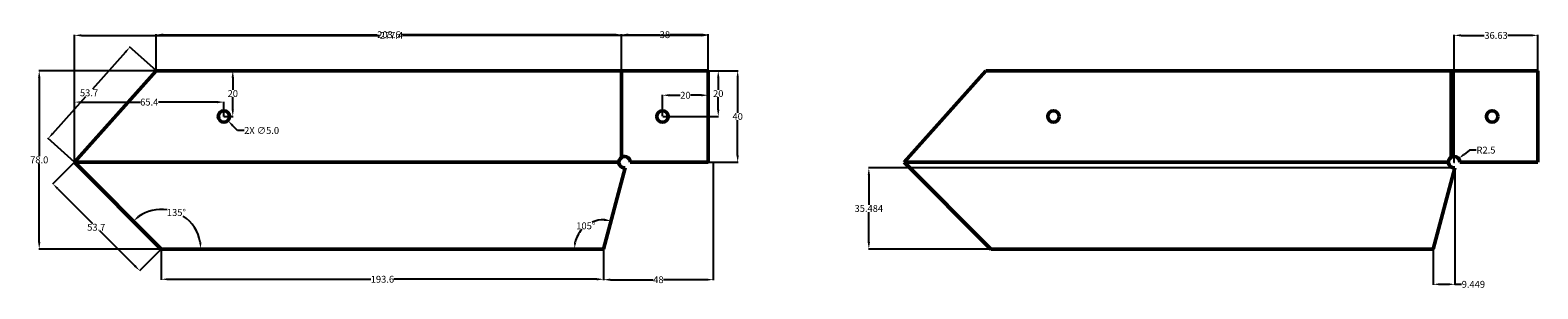
# Model space of a CAD drawing. Units: millimetres. Extents: x -38 to 622, y -14 to 99.
import ezdxf

# ---------------------------------------------------------------- set-up
doc = ezdxf.new("R2010")
doc.units = ezdxf.units.MM
doc.header["$MEASUREMENT"] = 0
doc.layers.add('M-DIMS', color=3, linetype='Continuous', lineweight=25)
doc.layers.add('M-OUTL', color=7, linetype='Continuous', lineweight=50)
doc.styles.get("Standard").update_dxf_attribs({"font": 'arial.ttf'})
doc.dimstyles.get("Standard").update_dxf_attribs({"dimtxt": 3, "dimasz": 3, "dimexe": 0.18, "dimexo": 0.0625, "dimgap": 0.09, "dimtad": 0, "dimtih": 1, "dimtoh": 1, "dimdec": 1, "dimdsep": 46, "dimtxsty": 'Standard', "dimcen": 0.09, "dimadec": 0, "dimazin": 0, "dimtfac": 1, "dimtdec": 1, "dimtofl": 0, "dimtmove": 0, "dimatfit": 3, "dimfxl": 1, "dimtolj": 1, "dimtzin": 0, "dimarcsym": 0})

# ---------------------------------------------------------------- blocks, each defined once
blk = doc.blocks.new('*D1')
at = {"layer": 'Defpoints', "color": 0, "transparency": 16777216}
for p in [(227.37, 56.06), (208.92, 15.24), (19.7, 3.24), (213.3, 3.24), (213.3, 3.24)]:
    blk.add_point(p, dxfattribs=at)
at = {"layer": 'M-DIMS', "color": 0, "lineweight": -2, "transparency": 16777216}
for start, end in [(88.5716, 113.10406), (138.24338, 166.51731)]:
    blk.add_arc((213.3, 3.24), 12.78, start, end, dxfattribs=at)
at = {"layer": 'M-DIMS', "color": 0, "transparency": 16777216}
for points in [[(213.69, 16.51), (213.55, 15.52), (216.59, 15.58)], [(201.37, 6.16), (200.38, 6.27), (200.53, 3.24)]]:
    blk.add_solid(points, dxfattribs=at)
at = {"layer": 'M-DIMS', "color": 0, "transparency": 16777216, "insert": (205.52, 13.37), "char_height": 3, "attachment_point": 5}
blk.add_mtext('\\A1;105°', dxfattribs=at)
blk = doc.blocks.new('*D2')
at = {"layer": 'Defpoints', "color": 0, "transparency": 16777216}
for p in [(19.7, 3.24), (213.3, 3.24), (213.3, -10)]:
    blk.add_point(p, dxfattribs=at)
at = {"layer": 'M-DIMS', "color": 0, "lineweight": -2, "transparency": 16777216}
for p, q in [((19.7, 3.17), (19.7, -10.18)), ((213.3, 3.17), (213.3, -10.18)), ((22.7, -10), (111.49, -10)), ((210.3, -10), (121.51, -10))]:
    blk.add_line(p, q, dxfattribs=at)
at = {"layer": 'M-DIMS', "color": 0, "transparency": 16777216}
for points in [[(22.7, -9.5), (22.7, -10.5), (19.7, -10)], [(210.3, -9.5), (210.3, -10.5), (213.3, -10)]]:
    blk.add_solid(points, dxfattribs=at)
at = {"layer": 'M-DIMS', "color": 0, "transparency": 16777216, "insert": (116.5, -10), "char_height": 3, "attachment_point": 5}
blk.add_mtext('\\A1;193.6', dxfattribs=at)
blk = doc.blocks.new('*D3')
at = {"layer": 'Defpoints', "color": 0, "transparency": 16777216}
for p in [(-18.27, 41.21), (19.7, 3.24), (10.23, -6.23)]:
    blk.add_point(p, dxfattribs=at)
at = {"layer": 'M-DIMS', "color": 0, "lineweight": -2, "transparency": 16777216}
for p, q in [((-18.31, 41.16), (-27.87, 31.61)), ((-25.62, 29.62), (-10.38, 14.38)), ((8.11, -4.11), (-7.13, 11.13)), ((19.66, 3.19), (10.11, -6.36))]:
    blk.add_line(p, q, dxfattribs=at)
at = {"layer": 'M-DIMS', "color": 0, "transparency": 16777216}
for points in [[(-25.26, 29.97), (-25.97, 29.26), (-27.74, 31.74)], [(8.47, -3.76), (7.76, -4.47), (10.23, -6.23)]]:
    blk.add_solid(points, dxfattribs=at)
at = {"layer": 'M-DIMS', "color": 0, "transparency": 16777216, "insert": (-8.75, 12.75), "char_height": 3, "attachment_point": 5}
blk.add_mtext('\\A1;53.7', dxfattribs=at)
blk = doc.blocks.new('*D4')
at = {"layer": 'Defpoints', "color": 0, "transparency": 16777216}
for p in [(5.98, 91.57), (17.53, 81.24), (-18.27, 41.21)]:
    blk.add_point(p, dxfattribs=at)
at = {"layer": 'M-DIMS', "color": 0, "lineweight": -2, "transparency": 16777216}
for p, q in [((3.98, 89.33), (-10.47, 73.17)), ((17.48, 81.28), (5.84, 91.69)), ((-27.82, 53.77), (-13.37, 69.93)), ((-18.31, 41.25), (-29.95, 51.66))]:
    blk.add_line(p, q, dxfattribs=at)
at = {"layer": 'M-DIMS', "color": 0, "transparency": 16777216}
for points in [[(3.6, 89.66), (4.35, 89), (5.98, 91.57)], [(-28.19, 54.11), (-27.45, 53.44), (-29.82, 51.54)]]:
    blk.add_solid(points, dxfattribs=at)
at = {"layer": 'M-DIMS', "color": 0, "transparency": 16777216, "insert": (-11.92, 71.55), "char_height": 3, "attachment_point": 5}
blk.add_mtext('\\A1;53.7', dxfattribs=at)
blk = doc.blocks.new('*D5')
at = {"layer": 'Defpoints', "color": 0, "transparency": 16777216}
for p in [(221.13, 97), (17.53, 81.24), (221.13, 81.24)]:
    blk.add_point(p, dxfattribs=at)
at = {"layer": 'M-DIMS', "color": 0, "lineweight": -2, "transparency": 16777216}
for p, q in [((17.53, 81.3), (17.53, 97.18)), ((20.53, 97), (114.15, 97)), ((218.13, 97), (124.5, 97)), ((221.13, 81.3), (221.13, 97.18))]:
    blk.add_line(p, q, dxfattribs=at)
at = {"layer": 'M-DIMS', "color": 0, "transparency": 16777216}
for points in [[(20.53, 97.5), (20.53, 96.5), (17.53, 97)], [(218.13, 97.5), (218.13, 96.5), (221.13, 97)]]:
    blk.add_solid(points, dxfattribs=at)
at = {"layer": 'M-DIMS', "color": 0, "transparency": 16777216, "insert": (119.33, 97), "char_height": 3, "attachment_point": 5}
blk.add_mtext('\\A1;203.6', dxfattribs=at)
blk = doc.blocks.new('*D6')
at = {"layer": 'Defpoints', "color": 0, "transparency": 16777216}
for p in [(259.13, 97), (221.13, 81.24), (259.13, 81.21)]:
    blk.add_point(p, dxfattribs=at)
at = {"layer": 'M-DIMS', "color": 0, "lineweight": -2, "transparency": 16777216}
for p, q in [((221.13, 81.3), (221.13, 97.18)), ((224.13, 97), (237.89, 97)), ((256.13, 97), (242.37, 97)), ((259.13, 81.27), (259.13, 97.18))]:
    blk.add_line(p, q, dxfattribs=at)
at = {"layer": 'M-DIMS', "color": 0, "transparency": 16777216}
for points in [[(224.13, 97.5), (224.13, 96.5), (221.13, 97)], [(256.13, 97.5), (256.13, 96.5), (259.13, 97)]]:
    blk.add_solid(points, dxfattribs=at)
at = {"layer": 'M-DIMS', "color": 0, "transparency": 16777216, "insert": (240.13, 97), "char_height": 3, "attachment_point": 5}
blk.add_mtext('\\A1;38', dxfattribs=at)
blk = doc.blocks.new('*D7')
at = {"layer": 'Defpoints', "color": 0, "transparency": 16777216}
for p in [(261.31, 41.21), (213.3, 3.24), (261.31, -10.18)]:
    blk.add_point(p, dxfattribs=at)
at = {"layer": 'M-DIMS', "color": 0, "lineweight": -2, "transparency": 16777216}
for p, q in [((261.31, 41.15), (261.31, -10.36)), ((213.3, 3.17), (213.3, -10.36)), ((216.3, -10.18), (235.01, -10.18)), ((258.31, -10.18), (239.61, -10.18))]:
    blk.add_line(p, q, dxfattribs=at)
at = {"layer": 'M-DIMS', "color": 0, "transparency": 16777216}
for points in [[(216.3, -9.68), (216.3, -10.68), (213.3, -10.18)], [(258.31, -9.68), (258.31, -10.68), (261.31, -10.18)]]:
    blk.add_solid(points, dxfattribs=at)
at = {"layer": 'M-DIMS', "color": 0, "transparency": 16777216, "insert": (237.31, -10.18), "char_height": 3, "attachment_point": 5}
blk.add_mtext('\\A1;48', dxfattribs=at)
blk = doc.blocks.new('*D8')
at = {"layer": 'Defpoints', "color": 0, "transparency": 16777216}
for p in [(-18.27, 41.21), (31.94, 15.47), (19.7, 3.24), (19.7, 3.24), (213.3, 3.24)]:
    blk.add_point(p, dxfattribs=at)
at = {"layer": 'M-DIMS', "color": 0, "lineweight": -2, "transparency": 16777216}
for start, end in [(81.47552, 125.05405), (9.94595, 56.10905)]:
    blk.add_arc((19.7, 3.24), 17.3, start, end, dxfattribs=at)
at = {"layer": 'M-DIMS', "color": 0, "transparency": 16777216}
for points in [[(10.09, 17.02), (9.44, 17.78), (7.47, 15.47)], [(37.25, 6.27), (36.25, 6.18), (37.01, 3.24)]]:
    blk.add_solid(points, dxfattribs=at)
at = {"layer": 'M-DIMS', "color": 0, "transparency": 16777216, "insert": (26.33, 19.22), "char_height": 3, "attachment_point": 5}
blk.add_mtext('\\A1;135°', dxfattribs=at)
blk = doc.blocks.new('*D9')
at = {"layer": 'Defpoints', "color": 0, "transparency": 16777216}
for p in [(259.13, 81.21), (272, 81.21), (259.13, 41.21)]:
    blk.add_point(p, dxfattribs=at)
at = {"layer": 'M-DIMS', "color": 0, "lineweight": -2, "transparency": 16777216}
for p, q in [((259.19, 81.21), (272.18, 81.21)), ((272, 78.21), (272, 62.83)), ((272, 44.21), (272, 59.59)), ((259.19, 41.21), (272.18, 41.21))]:
    blk.add_line(p, q, dxfattribs=at)
at = {"layer": 'M-DIMS', "color": 0, "transparency": 16777216}
for points in [[(271.5, 78.21), (272.5, 78.21), (272, 81.21)], [(271.5, 44.21), (272.5, 44.21), (272, 41.21)]]:
    blk.add_solid(points, dxfattribs=at)
at = {"layer": 'M-DIMS', "color": 0, "transparency": 16777216, "insert": (272, 61.21), "char_height": 3, "attachment_point": 5}
blk.add_mtext('\\A1;40', dxfattribs=at)
blk = doc.blocks.new('*D10')
at = {"layer": 'Defpoints', "color": 0, "transparency": 16777216}
for p in [(259.13, 81.21), (263.5, 81.21), (239.13, 61.23)]:
    blk.add_point(p, dxfattribs=at)
at = {"layer": 'M-DIMS', "color": 0, "lineweight": -2, "transparency": 16777216}
for p, q in [((259.19, 81.21), (263.68, 81.21)), ((263.5, 78.21), (263.5, 72.84)), ((263.5, 64.23), (263.5, 69.6)), ((239.19, 61.23), (263.68, 61.23))]:
    blk.add_line(p, q, dxfattribs=at)
at = {"layer": 'M-DIMS', "color": 0, "transparency": 16777216}
for points in [[(263, 78.21), (264, 78.21), (263.5, 81.21)], [(263, 64.23), (264, 64.23), (263.5, 61.23)]]:
    blk.add_solid(points, dxfattribs=at)
at = {"layer": 'M-DIMS', "color": 0, "transparency": 16777216, "insert": (263.5, 71.22), "char_height": 3, "attachment_point": 5}
blk.add_mtext('\\A1;20', dxfattribs=at)
blk = doc.blocks.new('*D11')
at = {"layer": 'Defpoints', "color": 0, "transparency": 16777216}
for p in [(259.13, 70.5), (239.13, 61.23), (259.13, 61.23)]:
    blk.add_point(p, dxfattribs=at)
at = {"layer": 'M-DIMS', "color": 0, "lineweight": -2, "transparency": 16777216}
for p, q in [((239.13, 61.29), (239.13, 70.68)), ((242.13, 70.5), (246.87, 70.5)), ((256.13, 70.5), (251.39, 70.5)), ((259.13, 61.29), (259.13, 70.68))]:
    blk.add_line(p, q, dxfattribs=at)
at = {"layer": 'M-DIMS', "color": 0, "transparency": 16777216}
for points in [[(242.13, 71), (242.13, 70), (239.13, 70.5)], [(256.13, 71), (256.13, 70), (259.13, 70.5)]]:
    blk.add_solid(points, dxfattribs=at)
at = {"layer": 'M-DIMS', "color": 0, "transparency": 16777216, "insert": (249.13, 70.5), "char_height": 3, "attachment_point": 5}
blk.add_mtext('\\A1;20', dxfattribs=at)
blk = doc.blocks.new('*D12')
at = {"layer": 'Defpoints', "color": 0, "transparency": 16777216}
for p in [(47.13, 67.5), (47.13, 61.24), (-18.27, 41.21)]:
    blk.add_point(p, dxfattribs=at)
at = {"layer": 'M-DIMS', "color": 0, "lineweight": -2, "transparency": 16777216}
for p, q in [((-18.27, 41.27), (-18.27, 67.68)), ((-15.27, 67.5), (10.44, 67.5)), ((44.13, 67.5), (18.42, 67.5)), ((47.13, 61.3), (47.13, 67.68))]:
    blk.add_line(p, q, dxfattribs=at)
at = {"layer": 'M-DIMS', "color": 0, "transparency": 16777216}
for points in [[(-15.27, 68), (-15.27, 67), (-18.27, 67.5)], [(44.13, 68), (44.13, 67), (47.13, 67.5)]]:
    blk.add_solid(points, dxfattribs=at)
at = {"layer": 'M-DIMS', "color": 0, "transparency": 16777216, "insert": (14.43, 67.5), "char_height": 3, "attachment_point": 5}
blk.add_mtext('\\A1;65.4', dxfattribs=at)
blk = doc.blocks.new('*D13')
at = {"layer": 'Defpoints', "color": 0, "transparency": 16777216}
for p in [(47.13, 81.24), (51, 81.24), (47.13, 61.24)]:
    blk.add_point(p, dxfattribs=at)
at = {"layer": 'M-DIMS', "color": 0, "lineweight": -2, "transparency": 16777216}
for p, q in [((47.19, 81.24), (51.18, 81.24)), ((51, 78.24), (51, 72.86)), ((51, 64.24), (51, 69.62)), ((47.19, 61.24), (51.18, 61.24))]:
    blk.add_line(p, q, dxfattribs=at)
at = {"layer": 'M-DIMS', "color": 0, "transparency": 16777216}
for points in [[(50.5, 78.24), (51.5, 78.24), (51, 81.24)], [(50.5, 64.24), (51.5, 64.24), (51, 61.24)]]:
    blk.add_solid(points, dxfattribs=at)
at = {"layer": 'M-DIMS', "color": 0, "transparency": 16777216, "insert": (51, 71.24), "char_height": 3, "attachment_point": 5}
blk.add_mtext('\\A1;20', dxfattribs=at)
blk = doc.blocks.new('POINTED-MOUNTING-PLATE')
for p, q in [((0, 37.97), (35.79, 78)), ((239.39, 78), (35.79, 78)), ((239.39, 78), (239.39, 40.06)), ((277.39, 77.97), (239.39, 77.97)), ((277.39, 37.97), (277.39, 77.97)), ((37.97, 0), (0, 37.97)), ((0, 37.97), (238.27, 37.97)), ((231.57, 0), (241.02, 35.48)), ((243.27, 37.97), (277.39, 37.97)), ((37.97, 0), (231.57, 0))]:
    blk.add_line(p, q)
for centre in [(65.4, 58), (257.39, 57.99)]:
    blk.add_circle(centre, 2.5)
blk.add_arc((240.77, 37.97), 2.5, 0, 275.793)
blk = doc.blocks.new('*D15')
at = {"layer": 'Defpoints', "color": 0, "transparency": 16777216}
for p in [(259.13, 96.69), (259.13, 81.21), (-18.27, 41.21)]:
    blk.add_point(p, dxfattribs=at)
at = {"layer": 'M-DIMS', "color": 0, "lineweight": -2, "transparency": 16777216}
for p, q in [((-18.27, 41.27), (-18.27, 96.87)), ((-15.27, 96.69), (115.26, 96.69)), ((256.13, 96.69), (125.6, 96.69)), ((259.13, 81.27), (259.13, 96.87))]:
    blk.add_line(p, q, dxfattribs=at)
at = {"layer": 'M-DIMS', "color": 0, "transparency": 16777216}
for points in [[(-15.27, 97.19), (-15.27, 96.19), (-18.27, 96.69)], [(256.13, 97.19), (256.13, 96.19), (259.13, 96.69)]]:
    blk.add_solid(points, dxfattribs=at)
at = {"layer": 'M-DIMS', "color": 0, "transparency": 16777216, "insert": (120.43, 96.69), "char_height": 3, "attachment_point": 5}
blk.add_mtext('\\A1;277.4', dxfattribs=at)
blk = doc.blocks.new('*D16')
at = {"layer": 'Defpoints', "color": 0, "transparency": 16777216}
for p in [(17.53, 81.24), (-33.72, 3.24), (19.7, 3.24)]:
    blk.add_point(p, dxfattribs=at)
at = {"layer": 'M-DIMS', "color": 0, "lineweight": -2, "transparency": 16777216}
for p, q in [((17.46, 81.24), (-33.9, 81.24)), ((-33.72, 78.24), (-33.72, 43.86)), ((-33.72, 6.24), (-33.72, 40.62)), ((19.64, 3.24), (-33.9, 3.24))]:
    blk.add_line(p, q, dxfattribs=at)
at = {"layer": 'M-DIMS', "color": 0, "transparency": 16777216}
for points in [[(-34.22, 78.24), (-33.22, 78.24), (-33.72, 81.24)], [(-34.22, 6.24), (-33.22, 6.24), (-33.72, 3.24)]]:
    blk.add_solid(points, dxfattribs=at)
at = {"layer": 'M-DIMS', "color": 0, "transparency": 16777216, "insert": (-33.72, 42.24), "char_height": 3, "attachment_point": 5}
blk.add_mtext('\\A1;78.0', dxfattribs=at)
blk = doc.blocks.new('*D17')
at = {"layer": 'Defpoints', "color": 0, "transparency": 16777216}
for p in [(585.89, 38.72), (576.44, 3.24), (585.89, -12.21)]:
    blk.add_point(p, dxfattribs=at)
at = {"layer": 'M-DIMS', "color": 0, "lineweight": -2, "transparency": 16777216}
for p, q in [((585.89, 38.66), (585.89, -12.39)), ((576.44, 3.17), (576.44, -12.39)), ((579.44, -12.21), (582.89, -12.21)), ((585.89, -12.21), (588.89, -12.21))]:
    blk.add_line(p, q, dxfattribs=at)
at = {"layer": 'M-DIMS', "color": 0, "transparency": 16777216}
for points in [[(579.44, -11.71), (579.44, -12.71), (576.44, -12.21)], [(582.89, -11.71), (582.89, -12.71), (585.89, -12.21)]]:
    blk.add_solid(points, dxfattribs=at)
at = {"layer": 'M-DIMS', "color": 0, "transparency": 16777216, "insert": (594.04, -12.21), "char_height": 3, "attachment_point": 5}
blk.add_mtext('\\A1;9.449', dxfattribs=at)
blk = doc.blocks.new('*D18')
at = {"layer": 'Defpoints', "color": 0, "transparency": 16777216}
for p in [(329.42, 38.72), (585.89, 38.72), (576.44, 3.24)]:
    blk.add_point(p, dxfattribs=at)
at = {"layer": 'M-DIMS', "color": 0, "lineweight": -2, "transparency": 16777216}
for p, q in [((585.82, 38.72), (329.24, 38.72)), ((329.42, 35.72), (329.42, 22.6)), ((329.42, 6.24), (329.42, 19.36)), ((576.37, 3.24), (329.24, 3.24))]:
    blk.add_line(p, q, dxfattribs=at)
at = {"layer": 'M-DIMS', "color": 0, "transparency": 16777216}
for points in [[(328.92, 35.72), (329.92, 35.72), (329.42, 38.72)], [(328.92, 6.24), (329.92, 6.24), (329.42, 3.24)]]:
    blk.add_solid(points, dxfattribs=at)
at = {"layer": 'M-DIMS', "color": 0, "transparency": 16777216, "insert": (329.42, 20.98), "char_height": 3, "attachment_point": 5}
blk.add_mtext('\\A1;35.484', dxfattribs=at)
blk = doc.blocks.new('*D19')
at = {"layer": 'Defpoints', "color": 0, "transparency": 16777216}
for p in [(622.26, 96.69), (622.26, 81.21), (585.63, 41.21)]:
    blk.add_point(p, dxfattribs=at)
at = {"layer": 'M-DIMS', "color": 0, "lineweight": -2, "transparency": 16777216}
for p, q in [((585.63, 41.27), (585.63, 96.87)), ((588.63, 96.69), (598.8, 96.69)), ((619.26, 96.69), (609.1, 96.69)), ((622.26, 81.27), (622.26, 96.87))]:
    blk.add_line(p, q, dxfattribs=at)
at = {"layer": 'M-DIMS', "color": 0, "transparency": 16777216}
for points in [[(588.63, 97.19), (588.63, 96.19), (585.63, 96.69)], [(619.26, 97.19), (619.26, 96.19), (622.26, 96.69)]]:
    blk.add_solid(points, dxfattribs=at)
at = {"layer": 'M-DIMS', "color": 0, "transparency": 16777216, "insert": (603.95, 96.69), "char_height": 3, "attachment_point": 5}
blk.add_mtext('\\A1;36.63', dxfattribs=at)
blk = doc.blocks.new('*D20')
at = {"layer": 'Defpoints', "color": 0, "transparency": 16777216}
for p in [(45.4, 63.05), (48.86, 59.43)]:
    blk.add_point(p, dxfattribs=at)
at = {"layer": 'M-DIMS', "color": 0, "lineweight": -2, "transparency": 16777216}
for p, q in [((47.04, 61.24), (47.22, 61.24)), ((47.13, 61.15), (47.13, 61.33)), ((53, 55.09), (50.93, 57.26)), ((56, 55.09), (53, 55.09))]:
    blk.add_line(p, q, dxfattribs=at)
at = {"layer": 'M-DIMS', "color": 0, "transparency": 16777216}
blk.add_solid([(51.29, 57.61), (50.57, 56.92), (48.86, 59.43)], dxfattribs=at)
at = {"layer": 'M-DIMS', "color": 0, "transparency": 16777216, "insert": (63.62, 55.09), "char_height": 3, "attachment_point": 5}
blk.add_mtext('\\A1;2X ∅5.0', dxfattribs=at)
blk = doc.blocks.new('*D21')
at = {"layer": 'Defpoints', "color": 0, "transparency": 16777216}
for p in [(585.63, 41.21), (587.59, 42.76)]:
    blk.add_point(p, dxfattribs=at)
at = {"layer": 'M-DIMS', "color": 0, "lineweight": -2, "transparency": 16777216}
for p, q in [((592.29, 46.5), (589.94, 44.63)), ((595.29, 46.5), (592.29, 46.5)), ((585.54, 41.21), (585.72, 41.21)), ((585.63, 41.12), (585.63, 41.3))]:
    blk.add_line(p, q, dxfattribs=at)
at = {"layer": 'M-DIMS', "color": 0, "transparency": 16777216}
blk.add_solid([(589.63, 45.02), (590.25, 44.24), (587.59, 42.76)], dxfattribs=at)
at = {"layer": 'M-DIMS', "color": 0, "transparency": 16777216, "insert": (599.56, 46.5), "char_height": 3, "attachment_point": 5}
blk.add_mtext('\\A1;R2.5', dxfattribs=at)

msp = doc.modelspace()

# ---------------------------------------------------------------- block references
at = {"layer": 'M-OUTL'}
for p in [(-18.268, 3.236), (344.8662, 3.236)]:
    msp.add_blockref('POINTED-MOUNTING-PLATE', p, dxfattribs=at)

# ---------------------------------------------------------------- dimensions: what is measured, and where the dimension line sits
at = {"layer": 'M-DIMS'}
for base, p1, p2, override, picture, middle in [((259.1268, 96.6881), (-18.2683, 41.2081), (259.1268, 81.2081), {"dimdec": 1, "dimlfac": 1, "dimrnd": 0, "dimzin": 0, "dimdsep": 46, "dimlunit": 2}, '*D15', (120.4292, 96.6881)), ((622.261, 96.6881), (585.6342, 41.2081), (622.261, 81.2081), {"dimdec": 2, "dimlfac": 1, "dimrnd": 0, "dimzin": 0, "dimdsep": 46, "dimlunit": 2}, '*D19', (603.9476, 96.6881)), ((585.8865, -12.2135), (576.4375, 3.2365), (585.8865, 38.7209), {"dimdec": 3, "dimlfac": 1, "dimrnd": 0, "dimzin": 0, "dimdsep": 46, "dimlunit": 2}, '*D17', (594.0413, -12.2135))]:
    dim = msp.add_linear_dim(base=base, p1=p1, p2=p2, dimstyle='Standard', override=override, dxfattribs=at)
    dim.commit()
    dim.dimension.update_dxf_attribs({"geometry": picture, "text_midpoint": middle})
at = {"layer": 'M-DIMS', "transparency": 33554610}
for base, p1, p2, picture, middle in [((221.1268, 97), (17.5268, 81.2381), (221.1268, 81.2381), '*D5', (119.3268, 97)), ((259.1268, 97), (221.1268, 81.2381), (259.1268, 81.2081), '*D6', (240.1268, 97)), ((47.1317, 67.5), (-18.2683, 41.2081), (47.1317, 61.2381), '*D12', (14.4317, 67.5)), ((259.1268, 70.5), (239.1268, 61.2271), (259.1268, 61.2271), '*D11', (249.1268, 70.5)), ((261.3147, -10.18), (213.3033, 3.2365), (261.3147, 41.2081), '*D7', (237.309, -10.18)), ((213.3033, -10), (19.7033, 3.2365), (213.3033, 3.2365), '*D2', (116.5033, -10))]:
    dim = msp.add_linear_dim(base=base, p1=p1, p2=p2, dimstyle='Standard', override={"dimclrd": 0, "dimclre": 0, "dimclrt": 0}, dxfattribs=at)
    dim.commit()
    dim.dimension.update_dxf_attribs({"geometry": picture, "text_midpoint": middle})
for p2, distance, picture, middle in [((17.5268, 81.2381), 15.4939, '*D4', (-11.9205, 71.5509)), ((19.7033, 3.2365), -13.3924, '*D3', (-8.7524, 12.7524))]:
    dim = msp.add_aligned_dim(p1=(-18.2683, 41.2081), p2=p2, distance=distance, dimstyle='Standard', override={"dimclrd": 0, "dimclre": 0, "dimclrt": 0}, dxfattribs=at)
    dim.commit()
    dim.dimension.update_dxf_attribs({"geometry": picture, "text_midpoint": middle})
at = {"layer": 'M-DIMS'}
for base, p1, p2, override, picture, middle in [((-33.7183, 3.2365), (17.5268, 81.2381), (19.7033, 3.2365), {"dimdec": 1, "dimlfac": 1, "dimrnd": 0, "dimzin": 0, "dimdsep": 46, "dimlunit": 2}, '*D16', (-33.7183, 42.2373)), ((329.4158, 38.7209), (576.4375, 3.2365), (585.8865, 38.7209), {"dimdec": 3, "dimlfac": 1, "dimrnd": 0, "dimzin": 0, "dimdsep": 46, "dimlunit": 2}, '*D18', (329.4158, 20.9787))]:
    dim = msp.add_linear_dim(base=base, p1=p1, p2=p2, angle=90, dimstyle='Standard', override=override, dxfattribs=at)
    dim.commit()
    dim.dimension.update_dxf_attribs({"geometry": picture, "text_midpoint": middle})
at = {"layer": 'M-DIMS', "transparency": 33554610}
for base, p1, p2, picture, middle in [((51, 81.2381), (47.1317, 61.2381), (47.1317, 81.2381), '*D13', (51, 71.2381)), ((263.5, 81.2081), (239.1268, 61.2271), (259.1268, 81.2081), '*D10', (263.5, 71.2176)), ((272, 81.2081), (259.1268, 41.2081), (259.1268, 81.2081), '*D9', (272, 61.2081))]:
    dim = msp.add_linear_dim(base=base, p1=p1, p2=p2, angle=90, dimstyle='Standard', override={"dimclrd": 0, "dimclre": 0, "dimclrt": 0}, dxfattribs=at)
    dim.commit()
    dim.dimension.update_dxf_attribs({"geometry": picture, "text_midpoint": middle})
at = {"layer": 'M-DIMS'}
dim = msp.add_diameter_dim_2p(p1=(45.4047, 63.0457), p2=(48.8587, 59.4305), text='2X <>', dimstyle='Standard', override={"dimdec": 1, "dimlfac": 1, "dimrnd": 0, "dimzin": 0, "dimdsep": 46, "dimlunit": 2}, dxfattribs=at)
dim.commit()
dim.dimension.update_dxf_attribs({"geometry": '*D20', "text_midpoint": (63.6201, 55.0922), "dimtype": 163})
at = {"layer": 'M-DIMS', "transparency": 33554610}
for base, line1, line2, picture, middle in [((208.9205, 15.2395), ((213.3033, 3.2365), (227.3693, 56.0592)), ((19.7033, 3.2365), (213.3033, 3.2365)), '*D1', (205.5166, 13.3681)), ((31.939, 15.4721), ((19.7033, 3.2365), (213.3033, 3.2365)), ((19.7033, 3.2365), (-18.2683, 41.2081)), '*D8', (26.3252, 19.2231))]:
    dim = msp.add_angular_dim_2l(base=base, line1=line1, line2=line2, dimstyle='Standard', override={"dimclrd": 0, "dimclre": 0, "dimclrt": 0}, dxfattribs=at)
    dim.commit()
    dim.dimension.update_dxf_attribs({"geometry": picture, "text_midpoint": middle})
at = {"layer": 'M-DIMS'}
dim = msp.add_radius_dim(center=(585.6342, 41.2081), mpoint=(587.5914, 42.7635), dimstyle='Standard', override={"dimdec": 1, "dimlfac": 1, "dimrnd": 0, "dimzin": 0, "dimdsep": 46, "dimlunit": 2}, dxfattribs=at)
dim.commit()
dim.dimension.update_dxf_attribs({"geometry": '*D21', "text_midpoint": (599.5565, 46.4963)})

doc.saveas('drawing.dxf')
